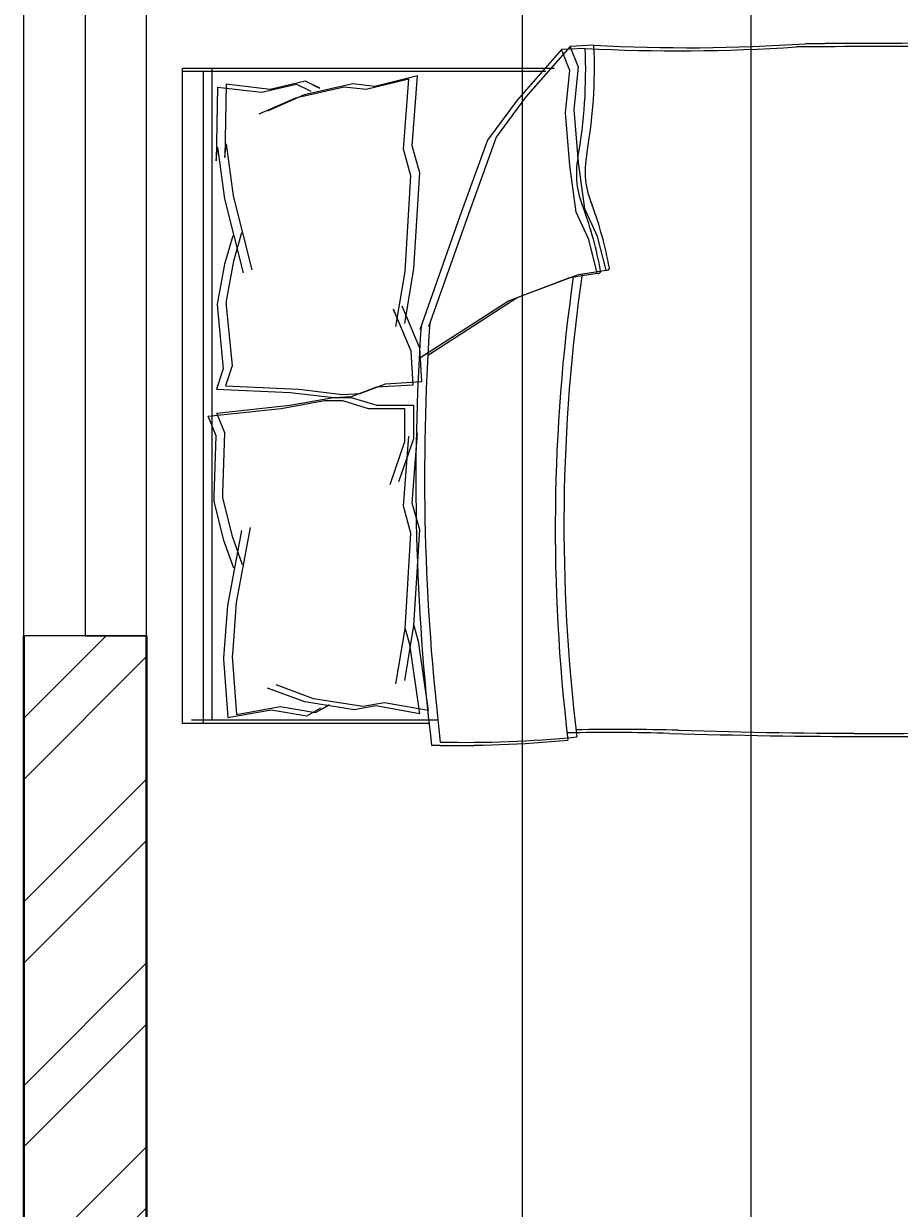
# Model space of a CAD drawing. Units: inches. Extents: x 1601 to 2297, y 1496 to 2631.
# Tile 39 of 57: x 1686 to 1750, y 2391 to 2478. Entities that reach past the tile are written whole.
import ezdxf

# ---------------------------------------------------------------- set-up
doc = ezdxf.new("R2010")
doc.units = ezdxf.units.IN
for name, color, linetype, lineweight in [('A-ANNO-DIMS', 2, 'Continuous', 18), ('A-FURN', 8, 'Continuous', 18), ('A-GLAZ', 161, 'Continuous', 20), ('A-WALL', 7, 'Continuous', 40), ('A-WALL-PATT', 215, 'Continuous', 13)]:
    doc.layers.add(name, color=color, linetype=linetype, lineweight=lineweight)
doc.styles.get("Standard").update_dxf_attribs({"font": 'arial.ttf'})
doc.dimstyles.get("Standard").update_dxf_attribs({"dimtxt": 0.18, "dimasz": 0.18, "dimexe": 0.18, "dimexo": 0.0625, "dimgap": 0.09, "dimtad": 0, "dimtih": 1, "dimtoh": 1, "dimdec": 4, "dimzin": 0, "dimdsep": 46, "dimtxsty": 'Standard', "dimcen": 0.09, "dimadec": 0, "dimazin": 0, "dimtfac": 1, "dimtdec": 4, "dimtofl": 0, "dimtmove": 0, "dimatfit": 3, "dimfxl": 1, "dimtolj": 1, "dimtzin": 0, "dimarcsym": 0})

# ---------------------------------------------------------------- blocks, each defined once
blk = doc.blocks.new('BED-DOUBLE')
for p, q in [((28.385, 53.096), (25.135, 49.39)), ((28.385, 53.096), (25.135, 49.39)), ((28.385, 53.096), (25.135, 49.39)), ((28.385, 53.096), (25.135, 49.39)), ((30.13, 53.175), (28.385, 53.096, 3.871)), ((30.13, 53.175), (28.385, 53.096, 3.871)), ((30.13, 53.175), (28.385, 53.096, 3.871)), ((30.13, 53.175), (28.385, 53.096, 3.871)), ((29.004, 51.559), (28.385, 53.096)), ((29.004, 51.558), (28.385, 53.096)), ((29.004, 51.559), (28.385, 53.096)), ((29.004, 51.558), (28.385, 53.096)), ((27.746, 52.867), (24.495, 49.162)), ((27.746, 52.867), (24.495, 49.162)), ((27.746, 52.867), (24.495, 49.162)), ((27.746, 52.867), (24.495, 49.162)), ((29.49, 52.947), (27.746, 52.867, 3.871)), ((29.49, 52.947), (27.746, 52.867, 3.871)), ((29.49, 52.947), (27.746, 52.867, 3.871)), ((29.49, 52.947), (27.746, 52.867, 3.871)), ((28.365, 51.33), (27.746, 52.867)), ((28.365, 51.33), (27.746, 52.867)), ((28.365, 51.33), (27.746, 52.867)), ((28.365, 51.33), (27.746, 52.867)), ((0, 51.494), (0.639, 51.493)), ((0, 3.475), (0, 51.494)), ((0, 51.494), (0.639, 51.493)), ((0, 3.475), (0, 51.494)), ((0, 51.265), (26.61, 51.265)), ((0, 51.265), (26.61, 51.265)), ((0, 51.265), (26.61, 51.265)), ((0, 51.265), (26.61, 51.265)), ((0.639, 51.494), (27.249, 51.494)), ((0.639, 51.494), (27.249, 51.494)), ((0.639, 51.493), (27.249, 51.493)), ((0.639, 51.493), (27.249, 51.493)), ((1.533, 3.475), (1.533, 51.265)), ((1.533, 3.475), (1.533, 51.265)), ((1.533, 3.475), (1.533, 51.265)), ((1.533, 3.475), (1.533, 51.265)), ((2.173, 3.703), (2.173, 51.494)), ((2.173, 3.703), (2.173, 51.494)), ((2.173, 3.703), (2.173, 51.493)), ((2.173, 3.703), (2.173, 51.493)), ((28.055, 48.233), (28.365, 51.33)), ((28.055, 48.233), (28.365, 51.33)), ((28.055, 48.233), (28.365, 51.33)), ((28.055, 48.233), (28.365, 51.33)), ((28.695, 48.461), (29.004, 51.559)), ((28.695, 48.461), (29.004, 51.559)), ((28.695, 48.461), (29.004, 51.558)), ((28.695, 48.461), (29.004, 51.558)), ((6.407, 49.961), (8.977, 50.557)), ((6.407, 49.961), (8.977, 50.557)), ((6.407, 49.961), (8.977, 50.556)), ((6.407, 49.961), (8.977, 50.556)), ((8.977, 50.557), (10.024, 50.043)), ((8.977, 50.557), (10.024, 50.043)), ((8.977, 50.556), (10.024, 50.042)), ((8.977, 50.556), (10.024, 50.042)), ((16.573, 50.698), (13.434, 49.923)), ((16.573, 50.698), (13.434, 49.922)), ((16.573, 50.698), (13.434, 49.923)), ((16.573, 50.698), (13.434, 49.922)), ((17.212, 50.926), (14.073, 50.151)), ((17.212, 50.926), (14.073, 50.151)), ((17.212, 50.926), (14.073, 50.151)), ((17.212, 50.926), (14.073, 50.151)), ((16.169, 45.566), (16.573, 50.698)), ((16.169, 45.566), (16.573, 50.698)), ((16.169, 45.566), (16.573, 50.698)), ((16.169, 45.566), (16.573, 50.698)), ((16.808, 45.795), (17.212, 50.926)), ((16.808, 45.794), (17.212, 50.926)), ((16.808, 45.795), (17.212, 50.926)), ((16.808, 45.794), (17.212, 50.926)), ((2.557, 50.112), (2.46, 44.709)), ((2.557, 50.112), (2.46, 44.709)), ((2.557, 50.111), (2.46, 44.709)), ((2.557, 50.111), (2.46, 44.709)), ((2.557, 50.112), (5.768, 49.733)), ((2.557, 50.112), (5.768, 49.733)), ((2.557, 50.111), (5.768, 49.733)), ((2.557, 50.111), (5.768, 49.733)), ((3.196, 50.34), (3.099, 44.938)), ((3.196, 50.34), (3.099, 44.938)), ((3.196, 50.34), (3.099, 44.938)), ((3.196, 50.34), (3.099, 44.938)), ((3.196, 50.34), (6.407, 49.961)), ((3.196, 50.34), (6.407, 49.961)), ((3.196, 50.34), (6.407, 49.961)), ((3.196, 50.34), (6.407, 49.961)), ((5.768, 49.733), (8.338, 50.328)), ((5.768, 49.733), (8.338, 50.328)), ((5.768, 49.733), (8.338, 50.328)), ((5.768, 49.733), (8.338, 50.328)), ((8.896, 49.538), (6.218, 48.356)), ((8.896, 49.538), (6.218, 48.356)), ((8.896, 49.537), (6.218, 48.356)), ((8.896, 49.537), (6.218, 48.356)), ((11.829, 50.112), (8.257, 49.309)), ((11.829, 50.112), (8.257, 49.309)), ((11.829, 50.112), (8.257, 49.309)), ((11.829, 50.112), (8.257, 49.309)), ((8.338, 50.328), (9.384, 49.814)), ((8.338, 50.328), (9.384, 49.814)), ((8.338, 50.328), (9.384, 49.814)), ((8.338, 50.328), (9.384, 49.814)), ((12.468, 50.34), (8.896, 49.538)), ((12.468, 50.34), (8.896, 49.537)), ((12.468, 50.34), (8.896, 49.538)), ((12.468, 50.34), (8.896, 49.537)), ((13.434, 49.923), (11.829, 50.112)), ((13.434, 49.922), (11.829, 50.112)), ((13.434, 49.923), (11.829, 50.112)), ((13.434, 49.922), (11.829, 50.112)), ((14.073, 50.151), (12.468, 50.34)), ((14.073, 50.151), (12.468, 50.34)), ((14.073, 50.151), (12.468, 50.34)), ((14.073, 50.151), (12.468, 50.34)), ((8.257, 49.309), (5.578, 48.128)), ((8.257, 49.309), (5.578, 48.128)), ((8.257, 49.309), (5.578, 48.128)), ((8.257, 49.309), (5.578, 48.128)), ((24.495, 49.162), (22.329, 46.219)), ((24.495, 49.162), (22.329, 46.219)), ((24.495, 49.162), (22.329, 46.219)), ((24.495, 49.162), (22.329, 46.219)), ((25.135, 49.39), (22.968, 46.448)), ((25.135, 49.39), (22.968, 46.448)), ((25.135, 49.39), (22.968, 46.448)), ((25.135, 49.39), (22.968, 46.448)), ((28.365, 44.361), (28.055, 48.233)), ((28.365, 44.361), (28.055, 48.233)), ((28.365, 44.361), (28.055, 48.233)), ((28.365, 44.361), (28.055, 48.233)), ((29.004, 44.589), (28.695, 48.461)), ((29.004, 44.589), (28.695, 48.461)), ((29.004, 44.589), (28.695, 48.461)), ((29.004, 44.589), (28.695, 48.461)), ((22.329, 46.219), (20.316, 40.644)), ((22.329, 46.219), (20.316, 40.644)), ((22.329, 46.219), (20.317, 40.644)), ((22.329, 46.219), (20.317, 40.644)), ((22.968, 46.448), (20.956, 40.872)), ((22.968, 46.448), (20.956, 40.872)), ((22.968, 46.448), (20.956, 40.872)), ((22.968, 46.448), (20.956, 40.872)), ((2.46, 44.709), (2.542, 45.712)), ((2.46, 44.709), (2.542, 45.712)), ((2.46, 44.709), (2.542, 45.712)), ((2.46, 44.709), (2.542, 45.712)), ((2.542, 45.712), (3.069, 41.914)), ((2.542, 45.712), (3.069, 41.914)), ((2.542, 45.712), (3.069, 41.914)), ((2.542, 45.712), (3.069, 41.914)), ((3.099, 44.938), (3.181, 45.941)), ((3.099, 44.938), (3.181, 45.941)), ((3.099, 44.938), (3.181, 45.94)), ((3.099, 44.938), (3.181, 45.94)), ((3.181, 45.941), (3.709, 42.143)), ((3.181, 45.941), (3.709, 42.143)), ((3.181, 45.94), (3.709, 42.142)), ((3.181, 45.94), (3.709, 42.142)), ((16.726, 43.606), (16.169, 45.566)), ((16.726, 43.606), (16.169, 45.566)), ((16.726, 43.606), (16.169, 45.566)), ((16.726, 43.606), (16.169, 45.566)), ((17.365, 43.834), (16.808, 45.795)), ((17.365, 43.834), (16.808, 45.795)), ((17.365, 43.834), (16.808, 45.794)), ((17.365, 43.834), (16.808, 45.794)), ((28.829, 40.954), (28.365, 44.361)), ((28.829, 40.953), (28.365, 44.361)), ((28.829, 40.954), (28.365, 44.361)), ((28.829, 40.953), (28.365, 44.361)), ((29.468, 41.182), (29.004, 44.589)), ((29.469, 41.182), (29.004, 44.589)), ((29.468, 41.182), (29.004, 44.589)), ((29.469, 41.182), (29.004, 44.589)), ((16.295, 36.596), (16.726, 43.606)), ((16.295, 36.596), (16.726, 43.606)), ((16.295, 36.596), (16.726, 43.606)), ((16.295, 36.596), (16.726, 43.606)), ((16.934, 36.824), (17.365, 43.834)), ((16.934, 36.824), (17.365, 43.834)), ((16.934, 36.824), (17.365, 43.834)), ((16.934, 36.824), (17.365, 43.834)), ((3.069, 41.914), (4.422, 36.495)), ((3.069, 41.914), (4.422, 36.495)), ((3.069, 41.914), (4.422, 36.495)), ((3.069, 41.914), (4.422, 36.495)), ((3.709, 42.143), (5.061, 36.723)), ((3.709, 42.143), (5.061, 36.723)), ((3.709, 42.142), (5.061, 36.723)), ((3.709, 42.142), (5.061, 36.723)), ((20.956, 40.872), (18.022, 32.534)), ((20.956, 40.872), (18.022, 32.534)), ((20.956, 40.872), (18.022, 32.534)), ((20.956, 40.872), (18.022, 32.534)), ((29.758, 38.94), (28.829, 40.954)), ((29.758, 38.94), (28.829, 40.954)), ((29.758, 38.94), (28.829, 40.953)), ((29.758, 38.94), (28.829, 40.953)), ((30.397, 39.169), (29.468, 41.182)), ((30.397, 39.169), (29.468, 41.182)), ((30.397, 39.168), (29.469, 41.182)), ((30.397, 39.168), (29.469, 41.182)), ((20.316, 40.644), (17.383, 32.306)), ((20.317, 40.644), (17.383, 32.306)), ((20.316, 40.644), (17.383, 32.306)), ((20.317, 40.644), (17.383, 32.306)), ((3.673, 39.2), (3.078, 37.135)), ((3.673, 39.2), (3.078, 37.135)), ((3.673, 39.2), (3.078, 37.135)), ((3.673, 39.2), (3.078, 37.135)), ((4.313, 39.428), (3.717, 37.363)), ((4.313, 39.428), (3.717, 37.363)), ((4.313, 39.428), (3.718, 37.363)), ((4.313, 39.428), (3.718, 37.363)), ((31.016, 36.691), (30.397, 39.169)), ((31.016, 36.691), (30.397, 39.169)), ((31.016, 36.691), (30.397, 39.168)), ((31.016, 36.691), (30.397, 39.168)), ((30.377, 36.462), (29.758, 38.94)), ((30.377, 36.462), (29.758, 38.94)), ((30.377, 36.462), (29.758, 38.94)), ((30.377, 36.462), (29.758, 38.94)), ((3.717, 37.363), (3.176, 34.433)), ((3.718, 37.363), (3.176, 34.433)), ((3.717, 37.363), (3.176, 34.433)), ((3.718, 37.363), (3.176, 34.433)), ((3.078, 37.135), (2.537, 34.204)), ((3.078, 37.135), (2.537, 34.204)), ((3.078, 37.135), (2.537, 34.204)), ((3.078, 37.135), (2.537, 34.204)), ((15.628, 32.564), (16.295, 36.596)), ((15.628, 32.564), (16.295, 36.596)), ((15.628, 32.564), (16.295, 36.596)), ((15.628, 32.564), (16.295, 36.596)), ((16.268, 32.792), (16.934, 36.824)), ((16.268, 32.792), (16.934, 36.824)), ((16.268, 32.792), (16.934, 36.824)), ((16.268, 32.792), (16.934, 36.824)), ((29.004, 36.381), (31.016, 36.691)), ((29.004, 36.381), (31.016, 36.691)), ((29.004, 36.381), (31.016, 36.691)), ((29.004, 36.381), (31.016, 36.691)), ((23.876, 34.449), (28.365, 36.153)), ((23.876, 34.449), (28.365, 36.153)), ((23.876, 34.449), (28.365, 36.152)), ((23.876, 34.449), (28.365, 36.152)), ((24.516, 34.677), (29.004, 36.381)), ((24.516, 34.677), (29.004, 36.381)), ((24.516, 34.677), (29.004, 36.381)), ((24.516, 34.677), (29.004, 36.381)), ((28.365, 36.153), (30.377, 36.462)), ((28.365, 36.152), (30.377, 36.462)), ((28.365, 36.153), (30.377, 36.462)), ((28.365, 36.152), (30.377, 36.462)), ((2.537, 34.204), (2.557, 33.883)), ((2.537, 34.204), (2.557, 33.883)), ((2.537, 34.204), (2.557, 33.883)), ((2.537, 34.204), (2.557, 33.883)), ((2.557, 33.883), (2.979, 29.456)), ((2.557, 33.883), (2.979, 29.455)), ((2.557, 33.883), (2.979, 29.456)), ((2.557, 33.883), (2.979, 29.455)), ((3.176, 34.433), (3.196, 34.112)), ((3.176, 34.433), (3.196, 34.112)), ((3.176, 34.433), (3.196, 34.112)), ((3.176, 34.433), (3.196, 34.112)), ((3.196, 34.112), (3.618, 29.684)), ((3.196, 34.112), (3.618, 29.684)), ((3.196, 34.112), (3.618, 29.684)), ((3.196, 34.112), (3.618, 29.684)), ((17.379, 30.978), (16.094, 34.049)), ((17.379, 30.978), (16.094, 34.049)), ((17.379, 30.978), (16.094, 34.049)), ((17.379, 30.978), (16.094, 34.049)), ((17.383, 30.259), (23.876, 34.449)), ((17.383, 30.259), (23.876, 34.449)), ((17.383, 30.259), (23.876, 34.449)), ((17.383, 30.259), (23.876, 34.449)), ((18.022, 30.487), (24.516, 34.677)), ((18.022, 30.487), (24.516, 34.677)), ((18.022, 30.487), (24.516, 34.677)), ((18.022, 30.487), (24.516, 34.677)), ((16.739, 30.75), (15.454, 33.821)), ((16.739, 30.75), (15.454, 33.821)), ((16.739, 30.75), (15.454, 33.82)), ((16.739, 30.75), (15.454, 33.82)), ((16.893, 28.297), (16.739, 30.75)), ((16.893, 28.297), (16.739, 30.75)), ((16.893, 28.297), (16.739, 30.75)), ((16.893, 28.297), (16.739, 30.75)), ((17.532, 28.526), (17.379, 30.978)), ((17.532, 28.525), (17.379, 30.978)), ((17.532, 28.526), (17.379, 30.978)), ((17.532, 28.525), (17.379, 30.978)), ((3.618, 29.684), (3.131, 28.205)), ((3.618, 29.684), (3.131, 28.205)), ((3.618, 29.684), (3.131, 28.205)), ((3.618, 29.684), (3.131, 28.205)), ((2.979, 29.456), (2.492, 27.977)), ((2.979, 29.456), (2.492, 27.977)), ((2.979, 29.455), (2.492, 27.976)), ((2.979, 29.455), (2.492, 27.976)), ((2.492, 27.977), (7.867, 27.733)), ((2.492, 27.977), (7.867, 27.733)), ((2.492, 27.976), (7.867, 27.733)), ((2.492, 27.976), (7.867, 27.733)), ((3.131, 28.205), (8.506, 27.962)), ((3.131, 28.205), (8.506, 27.961)), ((3.131, 28.205), (8.506, 27.962)), ((3.131, 28.205), (8.506, 27.961)), ((8.506, 27.962), (11.717, 27.583)), ((8.506, 27.962), (11.717, 27.583)), ((8.506, 27.961), (11.717, 27.583)), ((8.506, 27.961), (11.717, 27.583)), ((12.377, 27.436), (14.216, 28.13)), ((12.377, 27.436), (14.217, 28.13)), ((12.377, 27.436), (14.216, 28.13)), ((12.377, 27.436), (14.217, 28.13)), ((13.016, 27.664), (14.856, 28.359)), ((13.016, 27.664), (14.856, 28.359)), ((13.016, 27.664), (14.856, 28.358)), ((13.016, 27.664), (14.856, 28.358)), ((14.216, 28.13), (16.893, 28.297)), ((14.216, 28.13), (16.893, 28.297)), ((14.217, 28.13), (16.893, 28.297)), ((14.217, 28.13), (16.893, 28.297)), ((14.856, 28.359), (17.532, 28.526)), ((14.856, 28.359), (17.532, 28.526)), ((14.856, 28.358), (17.532, 28.525)), ((14.856, 28.358), (17.532, 28.525)), ((7.22, 26.561), (10.401, 27.139)), ((7.22, 26.56), (10.401, 27.139)), ((7.22, 26.561), (10.401, 27.139)), ((7.22, 26.56), (10.401, 27.139)), ((7.859, 26.789), (11.04, 27.367)), ((7.859, 26.789), (11.04, 27.367)), ((7.859, 26.789), (11.04, 27.367)), ((7.859, 26.789), (11.04, 27.367)), ((7.867, 27.733), (11.078, 27.355)), ((7.867, 27.733), (11.078, 27.354)), ((7.867, 27.733), (11.078, 27.355)), ((7.867, 27.733), (11.078, 27.354)), ((10.401, 27.139), (11.702, 27.139)), ((10.401, 27.139), (11.702, 27.139)), ((10.401, 27.139), (11.702, 27.139)), ((10.401, 27.139), (11.702, 27.139)), ((11.04, 27.367), (12.341, 27.367)), ((11.04, 27.367), (12.341, 27.367)), ((11.04, 27.367), (12.341, 27.367)), ((11.04, 27.367), (12.341, 27.367)), ((11.078, 27.355), (12.377, 27.436)), ((11.078, 27.354), (12.377, 27.436)), ((11.078, 27.355), (12.377, 27.436)), ((11.078, 27.354), (12.377, 27.436)), ((11.702, 27.139), (13.582, 26.561)), ((11.702, 27.139), (13.582, 26.56)), ((11.702, 27.139), (13.582, 26.561)), ((11.702, 27.139), (13.582, 26.56)), ((11.717, 27.583), (13.016, 27.664)), ((11.717, 27.583), (13.016, 27.664)), ((11.717, 27.583), (13.016, 27.664)), ((11.717, 27.583), (13.016, 27.664)), ((12.341, 27.367), (14.221, 26.789)), ((12.341, 27.367), (14.221, 26.789)), ((12.341, 27.367), (14.221, 26.789)), ((12.341, 27.367), (14.221, 26.789)), ((1.87, 25.982), (7.22, 26.561)), ((1.87, 25.982), (7.22, 26.561)), ((1.87, 25.982), (7.22, 26.56)), ((1.87, 25.982), (7.22, 26.56)), ((2.509, 26.211), (7.859, 26.789)), ((2.509, 26.21), (7.859, 26.789)), ((2.509, 26.211), (7.859, 26.789)), ((2.509, 26.21), (7.859, 26.789)), ((3.088, 24.765), (2.509, 26.211)), ((3.088, 24.765), (2.509, 26.211)), ((3.088, 24.765), (2.509, 26.21)), ((3.088, 24.765), (2.509, 26.21)), ((13.582, 26.561), (16.263, 26.561)), ((13.582, 26.561), (16.263, 26.561)), ((13.582, 26.56), (16.263, 26.56)), ((13.582, 26.56), (16.263, 26.56)), ((14.221, 26.789), (16.902, 26.789)), ((14.221, 26.789), (16.902, 26.789)), ((14.221, 26.789), (16.902, 26.789)), ((14.221, 26.789), (16.902, 26.789)), ((16.263, 26.561), (16.263, 24.103)), ((16.263, 26.561), (16.263, 24.103)), ((16.263, 26.56), (16.263, 24.103)), ((16.263, 26.56), (16.263, 24.103)), ((16.902, 26.789), (16.902, 24.332)), ((16.902, 26.789), (16.902, 24.331)), ((16.902, 26.789), (16.902, 24.332)), ((16.902, 26.789), (16.902, 24.331)), ((2.448, 24.537), (1.87, 25.982)), ((2.448, 24.537), (1.87, 25.982)), ((2.448, 24.537), (1.87, 25.982)), ((2.448, 24.537), (1.87, 25.982)), ((2.304, 20.091), (2.448, 24.537)), ((2.304, 20.091), (2.448, 24.537)), ((2.304, 20.091), (2.448, 24.537)), ((2.304, 20.091), (2.448, 24.537)), ((2.943, 20.32), (3.088, 24.765)), ((2.943, 20.319), (3.088, 24.765)), ((2.943, 20.32), (3.088, 24.765)), ((2.943, 20.319), (3.088, 24.765)), ((16.902, 24.332), (15.811, 21.187)), ((16.902, 24.332), (15.811, 21.187)), ((16.902, 24.331), (15.811, 21.187)), ((16.902, 24.331), (15.811, 21.187)), ((16.169, 19.384), (16.573, 24.516)), ((16.169, 19.384), (16.573, 24.516)), ((16.169, 19.383), (16.573, 24.515)), ((16.169, 19.383), (16.573, 24.515)), ((16.808, 19.612), (17.212, 24.744)), ((16.808, 19.612), (17.212, 24.744)), ((16.808, 19.612), (17.212, 24.744)), ((16.808, 19.612), (17.212, 24.744)), ((16.263, 24.103), (15.172, 20.959)), ((16.263, 24.103), (15.172, 20.958)), ((16.263, 24.103), (15.172, 20.959)), ((16.263, 24.103), (15.172, 20.958)), ((2.304, 19.77), (2.304, 20.091)), ((2.304, 19.769), (2.304, 20.091)), ((2.304, 19.77), (2.304, 20.091)), ((2.304, 19.769), (2.304, 20.091)), ((2.943, 19.998), (2.943, 20.32)), ((2.943, 19.998), (2.943, 20.32)), ((2.943, 19.998), (2.943, 20.319)), ((2.943, 19.998), (2.943, 20.319)), ((3.666, 17.107), (2.943, 19.998)), ((3.666, 17.107), (2.943, 19.998)), ((3.666, 17.107), (2.943, 19.998)), ((3.666, 17.107), (2.943, 19.998)), ((3.027, 16.878), (2.304, 19.77)), ((3.027, 16.878), (2.304, 19.77)), ((3.027, 16.878), (2.304, 19.769)), ((3.027, 16.878), (2.304, 19.769)), ((16.726, 17.423), (16.169, 19.384)), ((16.726, 17.423), (16.169, 19.384)), ((16.726, 17.423), (16.169, 19.383)), ((16.726, 17.423), (16.169, 19.383)), ((17.365, 17.652), (16.808, 19.612)), ((17.365, 17.651), (16.808, 19.612)), ((17.365, 17.652), (16.808, 19.612)), ((17.365, 17.651), (16.808, 19.612)), ((3.316, 12.108), (4.328, 17.601)), ((3.316, 12.108), (4.328, 17.601)), ((3.316, 12.108), (4.328, 17.601)), ((3.316, 12.108), (4.328, 17.601)), ((3.955, 12.336), (4.967, 17.83)), ((3.955, 12.336), (4.967, 17.83)), ((3.955, 12.336), (4.967, 17.829)), ((3.955, 12.336), (4.967, 17.829)), ((16.295, 10.413), (16.726, 17.423)), ((16.295, 10.413), (16.726, 17.423)), ((16.295, 10.413), (16.726, 17.423)), ((16.295, 10.413), (16.726, 17.423)), ((16.934, 10.642), (17.365, 17.652)), ((16.934, 10.642), (17.365, 17.652)), ((16.934, 10.642), (17.365, 17.651)), ((16.934, 10.642), (17.365, 17.651)), ((3.75, 14.855), (3.027, 16.878)), ((3.75, 14.854), (3.027, 16.878)), ((3.75, 14.855), (3.027, 16.878)), ((3.75, 14.854), (3.027, 16.878)), ((4.389, 15.083), (3.666, 17.107)), ((4.389, 15.083), (3.666, 17.107)), ((4.389, 15.083), (3.666, 17.107)), ((4.389, 15.083), (3.666, 17.107)), ((3.666, 8.513), (3.955, 12.336)), ((3.666, 8.513), (3.955, 12.336)), ((3.666, 8.513), (3.955, 12.336)), ((3.666, 8.513), (3.955, 12.336)), ((3.027, 8.285), (3.316, 12.108)), ((3.027, 8.284), (3.316, 12.108)), ((3.027, 8.285), (3.316, 12.108)), ((3.027, 8.284), (3.316, 12.108)), ((16.268, 6.61), (16.934, 10.642)), ((16.268, 6.61), (16.934, 10.642)), ((16.268, 6.61), (16.934, 10.642)), ((16.268, 6.61), (16.934, 10.642)), ((16.934, 10.642), (17.257, 9.509)), ((16.934, 10.642), (17.257, 9.508)), ((16.934, 10.642), (17.257, 9.509)), ((16.934, 10.642), (17.257, 9.508)), ((15.628, 6.382), (16.295, 10.413)), ((15.628, 6.381), (16.295, 10.413)), ((15.628, 6.382), (16.295, 10.413)), ((15.628, 6.381), (16.295, 10.413)), ((16.295, 10.413), (16.618, 9.28)), ((16.295, 10.413), (16.618, 9.28)), ((16.295, 10.413), (16.618, 9.28)), ((16.295, 10.413), (16.618, 9.28)), ((16.618, 9.28), (17.341, 4.184)), ((16.618, 9.28), (17.341, 4.183)), ((16.618, 9.28), (17.341, 4.184)), ((16.618, 9.28), (17.341, 4.183)), ((17.257, 9.509), (17.98, 4.412)), ((17.257, 9.509), (17.98, 4.412)), ((17.257, 9.508), (17.98, 4.412)), ((17.257, 9.508), (17.98, 4.412)), ((3.009, 8.179), (3.027, 8.285)), ((3.009, 8.179), (3.027, 8.285)), ((3.009, 8.179), (3.027, 8.284)), ((3.009, 8.179), (3.027, 8.284)), ((3.338, 3.898), (3.009, 8.179)), ((3.338, 3.898), (3.009, 8.179)), ((3.338, 3.898), (3.009, 8.179)), ((3.338, 3.898), (3.009, 8.179)), ((3.648, 8.408), (3.666, 8.513)), ((3.648, 8.407), (3.666, 8.513)), ((3.648, 8.408), (3.666, 8.513)), ((3.648, 8.407), (3.666, 8.513)), ((3.977, 4.127), (3.648, 8.408)), ((3.977, 4.127), (3.648, 8.408)), ((3.977, 4.127), (3.648, 8.407)), ((3.977, 4.127), (3.648, 8.407)), ((9.594, 5.279), (6.847, 6.291)), ((9.594, 5.279), (6.847, 6.291)), ((9.594, 5.279), (6.847, 6.291)), ((9.594, 5.279), (6.847, 6.291)), ((8.955, 5.051), (6.208, 6.063)), ((8.955, 5.051), (6.208, 6.063)), ((8.955, 5.051), (6.208, 6.063)), ((8.955, 5.051), (6.208, 6.063)), ((13.209, 4.701), (9.594, 5.279)), ((13.209, 4.701), (9.594, 5.279)), ((13.209, 4.701), (9.594, 5.279)), ((13.209, 4.701), (9.594, 5.279)), ((3.316, 3.894), (6.497, 4.473)), ((3.316, 3.894), (6.497, 4.473)), ((3.316, 3.894), (6.497, 4.472)), ((3.316, 3.894), (6.497, 4.472)), ((3.955, 4.123), (7.136, 4.701)), ((3.955, 4.123), (7.136, 4.701)), ((3.955, 4.123), (7.136, 4.701)), ((3.955, 4.123), (7.136, 4.701)), ((6.497, 4.473), (9.099, 4.039)), ((6.497, 4.473), (9.099, 4.039)), ((6.497, 4.472), (9.099, 4.039)), ((6.497, 4.472), (9.099, 4.039)), ((7.136, 4.701), (9.739, 4.267)), ((7.136, 4.701), (9.739, 4.267)), ((7.136, 4.701), (9.739, 4.267)), ((7.136, 4.701), (9.739, 4.267)), ((12.57, 4.473), (8.955, 5.051)), ((12.57, 4.472), (8.955, 5.051)), ((12.57, 4.473), (8.955, 5.051)), ((12.57, 4.472), (8.955, 5.051)), ((9.099, 4.039), (10.112, 4.617)), ((9.099, 4.039), (10.112, 4.617)), ((9.099, 4.039), (10.112, 4.617)), ((9.099, 4.039), (10.112, 4.617)), ((9.739, 4.267), (10.751, 4.846)), ((9.739, 4.267), (10.751, 4.846)), ((9.739, 4.267), (10.751, 4.845)), ((9.739, 4.267), (10.751, 4.845)), ((14.16, 4.762), (12.57, 4.473)), ((14.16, 4.762), (12.57, 4.472)), ((14.16, 4.762), (12.57, 4.473)), ((14.16, 4.762), (12.57, 4.472)), ((14.799, 4.99), (13.209, 4.701)), ((14.799, 4.99), (13.209, 4.701)), ((14.799, 4.99), (13.209, 4.701)), ((14.799, 4.99), (13.209, 4.701)), ((17.341, 4.184), (14.16, 4.762)), ((17.341, 4.183), (14.16, 4.762)), ((17.341, 4.184), (14.16, 4.762)), ((17.341, 4.183), (14.16, 4.762)), ((17.98, 4.412), (14.799, 4.99)), ((17.98, 4.412), (14.799, 4.99)), ((17.98, 4.412), (14.799, 4.99)), ((17.98, 4.412), (14.799, 4.99)), ((18.11, 3.475), (0, 3.475)), ((18.11, 3.475), (0, 3.475)), ((18.11, 3.475), (0, 3.475)), ((18.11, 3.475), (0, 3.475)), ((18.75, 3.703), (0.639, 3.703)), ((18.75, 3.703), (0.639, 3.703)), ((18.75, 3.703), (0.639, 3.703)), ((18.75, 3.703), (0.639, 3.703))]:
    blk.add_line(p, q)
for centre, radius, start, end in [((36.315, 182.266), 129.499, 266.97912, 273.83645), ((36.315, 182.265), 129.499, 266.97912, 273.83645), ((36.315, 182.266), 129.499, 266.97912, 273.83645), ((36.315, 182.265), 129.499, 266.97912, 273.83645), ((-6.017, 51.555), 36.183, 349.87628, 2.56571), ((-6.017, 51.555), 36.183, 349.87628, 2.56571), ((-6.017, 51.555), 36.183, 349.87628, 2.56571), ((-6.017, 51.555), 36.183, 349.87628, 2.56571), ((36.954, 182.494), 129.499, 266.97912, 273.83645), ((36.954, 182.494), 129.499, 266.97912, 273.83645), ((36.954, 182.494), 129.499, 266.97912, 273.83645), ((36.954, 182.494), 129.499, 266.97912, 273.83645), ((67.821, -4508.744), 4561.858, 90.002168, 90.286887), ((67.821, -4508.744), 4561.858, 90.002168, 90.286887), ((67.821, -4508.744), 4561.858, 90.002168, 90.286887), ((67.821, -4508.744), 4561.858, 90.002168, 90.286887), ((68.461, -4508.515), 4561.858, 90.002168, 90.286887), ((68.461, -4508.515), 4561.858, 90.002168, 90.286887), ((68.461, -4508.516), 4561.858, 90.002168, 90.286887), ((68.461, -4508.516), 4561.858, 90.002168, 90.286887), ((-6.656, 51.327), 36.183, 349.87628, 2.56571), ((-6.656, 51.327), 36.183, 349.87628, 2.56571), ((-6.656, 51.327), 36.183, 349.87628, 2.56571), ((-6.656, 51.327), 36.183, 349.87628, 2.56571), ((35.705, 43.972), 6.224, 168.6608, 203.73842), ((35.705, 43.971), 6.224, 168.6608, 203.73842), ((35.705, 43.972), 6.224, 168.6608, 203.73842), ((35.705, 43.971), 6.224, 168.6608, 203.73842), ((35.066, 43.743), 6.224, 168.6608, 203.73842), ((35.066, 43.743), 6.224, 168.6608, 203.73842), ((35.066, 43.743), 6.224, 168.6608, 203.73842), ((35.066, 43.743), 6.224, 168.6608, 203.73842), ((1.482, 31.154), 29.654, 10.66171, 19.88058), ((1.482, 31.154), 29.654, 10.66171, 19.88058), ((1.482, 31.153), 29.654, 10.66171, 19.88058), ((1.482, 31.153), 29.654, 10.66171, 19.88058), ((2.121, 31.382), 29.654, 10.66171, 19.88058), ((2.121, 31.382), 29.654, 10.66171, 19.88058), ((2.121, 31.382), 29.654, 10.66171, 19.88058), ((2.121, 31.382), 29.654, 10.66171, 19.88058), ((30.439, 36.636), 0.185, 250.24637, 1.13765), ((30.439, 36.636), 0.185, 250.24637, 1.13765), ((30.439, 36.636), 0.185, 250.24637, 1.13765), ((30.439, 36.636), 0.185, 250.24637, 1.13765), ((31.079, 36.864), 0.185, 250.24637, 1.13765), ((31.079, 36.864), 0.185, 250.24637, 1.13765), ((31.079, 36.864), 0.185, 250.24637, 1.13765), ((31.079, 36.864), 0.185, 250.24637, 1.13765), ((156.316, 17.756), 129.02, 171.78449, 186.90062), ((156.316, 17.755), 129.02, 171.78449, 186.90062), ((156.316, 17.756), 129.02, 171.78449, 186.90062), ((156.316, 17.755), 129.02, 171.78449, 186.90062), ((156.955, 17.984), 129.02, 171.78449, 186.90062), ((156.955, 17.984), 129.02, 171.78449, 186.90062), ((156.955, 17.984), 129.02, 171.78449, 186.90062), ((156.955, 17.984), 129.02, 171.78449, 186.90062), ((182.052, 21.359), 164.969, 176.08655, 186.78213), ((182.052, 21.359), 164.969, 176.08655, 186.78213), ((182.052, 21.358), 164.969, 176.08655, 186.78213), ((182.052, 21.358), 164.969, 176.08655, 186.78213), ((182.692, 21.587), 164.969, 176.08655, 186.78213), ((182.692, 21.587), 164.969, 176.08655, 186.78213), ((182.692, 21.587), 164.969, 176.08655, 186.78213), ((182.692, 21.587), 164.969, 176.08655, 186.78213), ((31.174, -167.308), 170.11, 88.4762, 91.00819), ((31.174, -167.308), 170.11, 88.4762, 91.00819), ((31.174, -167.308), 170.11, 88.4762, 91.00819), ((31.174, -167.308), 170.11, 88.4762, 91.00819), ((31.813, -167.079), 170.11, 88.4762, 91.00819), ((31.813, -167.08), 170.11, 88.4762, 91.00819), ((31.813, -167.079), 170.11, 88.4762, 91.00819), ((31.813, -167.08), 170.11, 88.4762, 91.00819), ((50.614, 484.822), 482.31, 268.22771, 271.71854), ((50.614, 484.822), 482.31, 268.22771, 271.71854), ((50.614, 484.822), 482.31, 268.22771, 271.71854), ((50.614, 484.822), 482.31, 268.22771, 271.71854), ((51.253, 485.051), 482.31, 268.22771, 271.71854), ((51.253, 485.05), 482.31, 268.22771, 271.71854), ((51.253, 485.051), 482.31, 268.22771, 271.71854), ((51.253, 485.05), 482.31, 268.22771, 271.71854), ((20.096, 85.162), 83.306, 268.72178, 275.60397), ((20.096, 85.161), 83.306, 268.72178, 275.60397), ((20.096, 85.162), 83.306, 268.72178, 275.60397), ((20.096, 85.161), 83.306, 268.72178, 275.60397), ((20.735, 85.39), 83.306, 268.72178, 275.60397), ((20.735, 85.39), 83.306, 268.72178, 275.60397), ((20.736, 85.39), 83.306, 268.72178, 275.60397), ((20.736, 85.39), 83.306, 268.72178, 275.60397)]:
    blk.add_arc(centre, radius, start, end)
blk = doc.blocks.new('WIN-60IN-JAMB9')
for p, q in [((4.5, 60), (0, 60)), ((0, 60), (9, 60)), ((0, 60), (0, 0)), ((4.5, 0), (4.5, 60)), ((9, 60), (9, 0)), ((0, 0), (9, 0)), ((9, 0), (4.5, 0))]:
    blk.add_line(p, q)
blk = doc.blocks.new('*D32')
at = {"layer": 'A-ANNO-DIMS', "color": 0, "lineweight": -2, "transparency": 16777216}
for p, q in [((1686.037, 2031.388), (1686.037, 2581.055)), ((1686.217, 2580.875), (1703.909, 2580.875)), ((1722.389, 2580.875), (1704.697, 2580.875)), ((1722.569, 2031.388), (1722.569, 2581.055))]:
    blk.add_line(p, q, dxfattribs=at)
at = {"layer": 'A-ANNO-DIMS', "color": 0, "transparency": 16777216}
for points in [[(1686.217, 2580.905), (1686.217, 2580.845), (1686.037, 2580.875)], [(1722.389, 2580.905), (1722.389, 2580.845), (1722.569, 2580.875)]]:
    blk.add_solid(points, dxfattribs=at)
at = {"layer": 'Defpoints', "color": 0, "transparency": 16777216}
for p in [(1722.569, 2580.875), (1686.037, 2031.325), (1722.569, 2031.325)]:
    blk.add_point(p, dxfattribs=at)
at = {"layer": 'A-ANNO-DIMS', "color": 0, "transparency": 16777216, "insert": (1704.303, 2580.875), "char_height": 0.18, "attachment_point": 5}
blk.add_mtext('\\A1;36.53', dxfattribs=at)
blk = doc.blocks.new('*D36')
at = {"layer": 'A-ANNO-DIMS', "color": 0, "lineweight": -2, "transparency": 16777216}
for p, q in [((1686.037, 1635.388), (1686.037, 2581.055)), ((1686.217, 2580.875), (1712.362, 2580.875)), ((1739.154, 2580.875), (1713.009, 2580.875)), ((1739.334, 1635.388), (1739.334, 2581.055))]:
    blk.add_line(p, q, dxfattribs=at)
at = {"layer": 'A-ANNO-DIMS', "color": 0, "transparency": 16777216}
for points in [[(1686.217, 2580.905), (1686.217, 2580.845), (1686.037, 2580.875)], [(1739.154, 2580.905), (1739.154, 2580.845), (1739.334, 2580.875)]]:
    blk.add_solid(points, dxfattribs=at)
at = {"layer": 'Defpoints', "color": 0, "transparency": 16777216}
for p in [(1739.334, 2580.875), (1686.037, 1635.325), (1739.334, 1635.325)]:
    blk.add_point(p, dxfattribs=at)
at = {"layer": 'A-ANNO-DIMS', "color": 0, "transparency": 16777216, "insert": (1712.685, 2580.875), "char_height": 0.18, "attachment_point": 5}
blk.add_mtext('\\A1;53.3', dxfattribs=at)

msp = doc.modelspace()

# ---------------------------------------------------------------- hatches: boundary and pattern name
at = {"layer": 'A-WALL-PATT'}
h = msp.add_hatch(dxfattribs=at)
h.set_pattern_fill('ANSI32', color=256)
h.paths.add_polyline_path([(1842.0336, 2528.0767), (1842.0336, 2532.3254), (1686.0373, 2532.3254), (1686.0373, 2492.9493), (1695.0373, 2492.9493), (1695.0373, 2523.3254), (1827.0373, 2523.3254), (1827.0373, 2416.8254), (1834.6225, 2416.8254), (1834.6225, 2419.0754), (1834.6225, 2421.3254), (1831.5373, 2421.3254), (1831.5373, 2523.3254), (1842.0336, 2523.3254)])
h.paths.add_polyline_path([(1695.0373, 2432.9493), (1686.0373, 2432.9493), (1686.0373, 2325.989), (1695.0373, 2325.989), (1695.0373, 2347.8254), (1827.0373, 2347.8254), (1827.0373, 2287.8254), (1823.2991, 2287.8254), (1823.2991, 2283.3254), (1847.9422, 2283.3254), (1847.9422, 2285.5754), (1847.9422, 2287.8254), (1831.5373, 2287.8254), (1831.5373, 2347.8254), (1846.9946, 2347.8254), (1846.9946, 2350.0754), (1846.9946, 2352.3254), (1695.0373, 2352.3254)])
h.paths.add_polyline_path([(1807.1169, 1573.5395), (2055.0405, 1573.5395), (2055.0405, 1610.6322), (1807.1169, 1610.6322)], flags=9)
h.paths.add_polyline_path([(1841.1631, 1712.7967), (1870.3957, 1712.7967), (1870.3957, 1731.454), (1841.1631, 1731.454)], flags=9)
h.paths.add_polyline_path([(2144.3862, 1772.185), (2191.0233, 1772.185), (2191.0233, 1790.8423), (2144.3862, 1790.8423)], flags=9)
h.paths.add_polyline_path([(2143.0128, 1827.3312), (2177.9958, 1827.3312), (2177.9958, 1845.9886), (2143.0128, 1845.9886)], flags=9)
h.paths.add_polyline_path([(2041.2439, 1833.5691), (2070.8516, 1833.5691), (2070.8516, 1852.2264), (2041.2439, 1852.2264)], flags=9)
h.paths.add_polyline_path([(2097.2791, 1947.0598), (2134.2061, 1947.0598), (2134.2061, 1965.7171), (2097.2791, 1965.7171)], flags=9)
h.paths.add_polyline_path([(2214.995, 1904.3124), (2214.995, 1942.2899), (2196.3376, 1942.2899), (2196.3376, 1904.3124)], flags=9)
h.paths.add_polyline_path([(2186.6284, 2043.8031), (2219.7935, 2043.8031), (2219.7935, 2062.4605), (2186.6284, 2062.4605)], flags=9)
h.paths.add_polyline_path([(2064.0877, 2031.616), (2097.4949, 2031.616), (2097.4949, 2050.2734), (2064.0877, 2050.2734)], flags=9)
h.paths.add_polyline_path([(1973.1349, 1986.0688), (2008.4009, 1986.0688), (2008.4009, 2004.7261), (1973.1349, 2004.7261)], flags=9)
h.paths.add_polyline_path([(1976.3676, 2106.9635), (2005.7469, 2106.9635), (2005.7469, 2125.6209), (1976.3676, 2125.6209)], flags=9)
h.paths.add_polyline_path([(1991.7852, 2180.4863), (2027.0513, 2180.4863), (2027.0513, 2199.1437), (1991.7852, 2199.1437)], flags=9)
h.paths.add_polyline_path([(2106.1801, 2187.9359), (2152.2101, 2187.9359), (2152.2101, 2206.5932), (2106.1801, 2206.5932)], flags=9)
h.paths.add_polyline_path([(2148.6686, 2262.2542), (2182.318, 2262.2542), (2182.318, 2280.9115), (2148.6686, 2280.9115)], flags=9)
h.paths.add_polyline_path([(2041.6327, 2252.8147), (2071.2405, 2252.8147), (2071.2405, 2271.4721), (2041.6327, 2271.4721)], flags=9)
h.paths.add_polyline_path([(2063.9734, 2375.4265), (2100.9004, 2375.4265), (2100.9004, 2394.0839), (2063.9734, 2394.0839)], flags=9)
h.paths.add_polyline_path([(2216.4955, 2330.9748), (2216.4955, 2370.2654), (2197.8381, 2370.2654), (2197.8381, 2330.9748)], flags=9)
h.paths.add_polyline_path([(2179.1416, 2485.8687), (2212.3067, 2485.8687), (2212.3067, 2504.5261), (2179.1416, 2504.5261)], flags=9)
h.paths.add_polyline_path([(2078.7442, 2471.1516), (2112.1514, 2471.1516), (2112.1514, 2489.809), (2078.7442, 2489.809)], flags=9)
h.paths.add_polyline_path([(1915.9631, 2329.4668), (1952.8902, 2329.4668), (1952.8902, 2348.1241), (1915.9631, 2348.1241)], flags=9)
h.paths.add_polyline_path([(1904.3189, 2499.6709), (1940.4512, 2499.6709), (1940.4512, 2518.3282), (1904.3189, 2518.3282)], flags=9)
h.paths.add_polyline_path([(1892.3665, 2100.4595), (1925.6374, 2100.4595), (1925.6374, 2119.1169), (1892.3665, 2119.1169)], flags=9)
h.paths.add_polyline_path([(1909.2984, 1805.9631), (1946.2254, 1805.9631), (1946.2254, 1824.6205), (1909.2984, 1824.6205)], flags=9)
h.paths.add_polyline_path([(1934.6056, 1658.616), (1970.738, 1658.616), (1970.738, 1677.2733), (1934.6056, 1677.2733)], flags=9)
h.paths.add_polyline_path([(1711.2052, 1789.8902), (1750.0456, 1789.8902), (1750.0456, 1808.5476), (1711.2052, 1808.5476)], flags=9)
h.paths.add_polyline_path([(1742.7874, 1854.6743), (1771.9449, 1854.6743), (1771.9449, 1873.3317), (1742.7874, 1873.3317)], flags=9)
h.paths.add_polyline_path([(1807.3592, 1997.7912), (1850.1116, 1997.7912), (1850.1116, 2016.4486), (1807.3592, 2016.4486)], flags=9)
h.paths.add_polyline_path([(1717.4579, 2237.7844), (1760.2103, 2237.7844), (1760.2103, 2256.4417), (1717.4579, 2256.4417)], flags=9)
h.paths.add_polyline_path([(1780.9285, 2324.0623), (1810.086, 2324.0623), (1810.086, 2342.7197), (1780.9285, 2342.7197)], flags=25)
h.paths.add_polyline_path([(1837.696, 2449.2024), (1866.9286, 2449.2024), (1866.9286, 2467.8598), (1837.696, 2467.8598)], flags=9)
h.paths.add_polyline_path([(1712.7752, 2484.9404), (1751.6156, 2484.9404), (1751.6156, 2503.5977), (1712.7752, 2503.5977)], flags=25)

# ---------------------------------------------------------------- linework, layer by layer
at = {"layer": 'A-WALL'}
for p, q in [((1686.0373, 2432.9493), (1686.0373, 2325.989)), ((1695.0373, 2432.9493), (1695.0373, 2352.3254))]:
    msp.add_line(p, q, dxfattribs=at)

# ---------------------------------------------------------------- block references
at = {"layer": 'A-FURN'}
msp.add_blockref('BED-DOUBLE', (1697.682, 2423.048), dxfattribs=at)
at = {"layer": 'A-GLAZ', "rotation": 180}
msp.add_blockref('WIN-60IN-JAMB9', (1695.0376, 2492.9498), dxfattribs=at)

# ---------------------------------------------------------------- dimensions: what is measured, and where the dimension line sits
at = {"layer": 'A-ANNO-DIMS'}
for base, p1, p2, override, picture, middle in [((1722.5687, 2580.8754), (1686.0373, 2031.3254), (1722.5687, 2031.3254), {"dimdec": 2, "dimlfac": 1, "dimrnd": 0, "dimzin": 0, "dimdsep": 46, "dimlunit": 2}, '*D32', (1704.303, 2580.8754)), ((1739.3335, 2580.8754), (1686.0373, 1635.3254), (1739.3335, 1635.3254), {"dimdec": 1, "dimlfac": 1, "dimrnd": 0, "dimzin": 0, "dimdsep": 46, "dimlunit": 2}, '*D36', (1712.6854, 2580.8754))]:
    dim = msp.add_linear_dim(base=base, p1=p1, p2=p2, dimstyle='Standard', override=override, dxfattribs=at)
    dim.commit()
    dim.dimension.update_dxf_attribs({"geometry": picture, "text_midpoint": middle})

doc.saveas('drawing.dxf')
